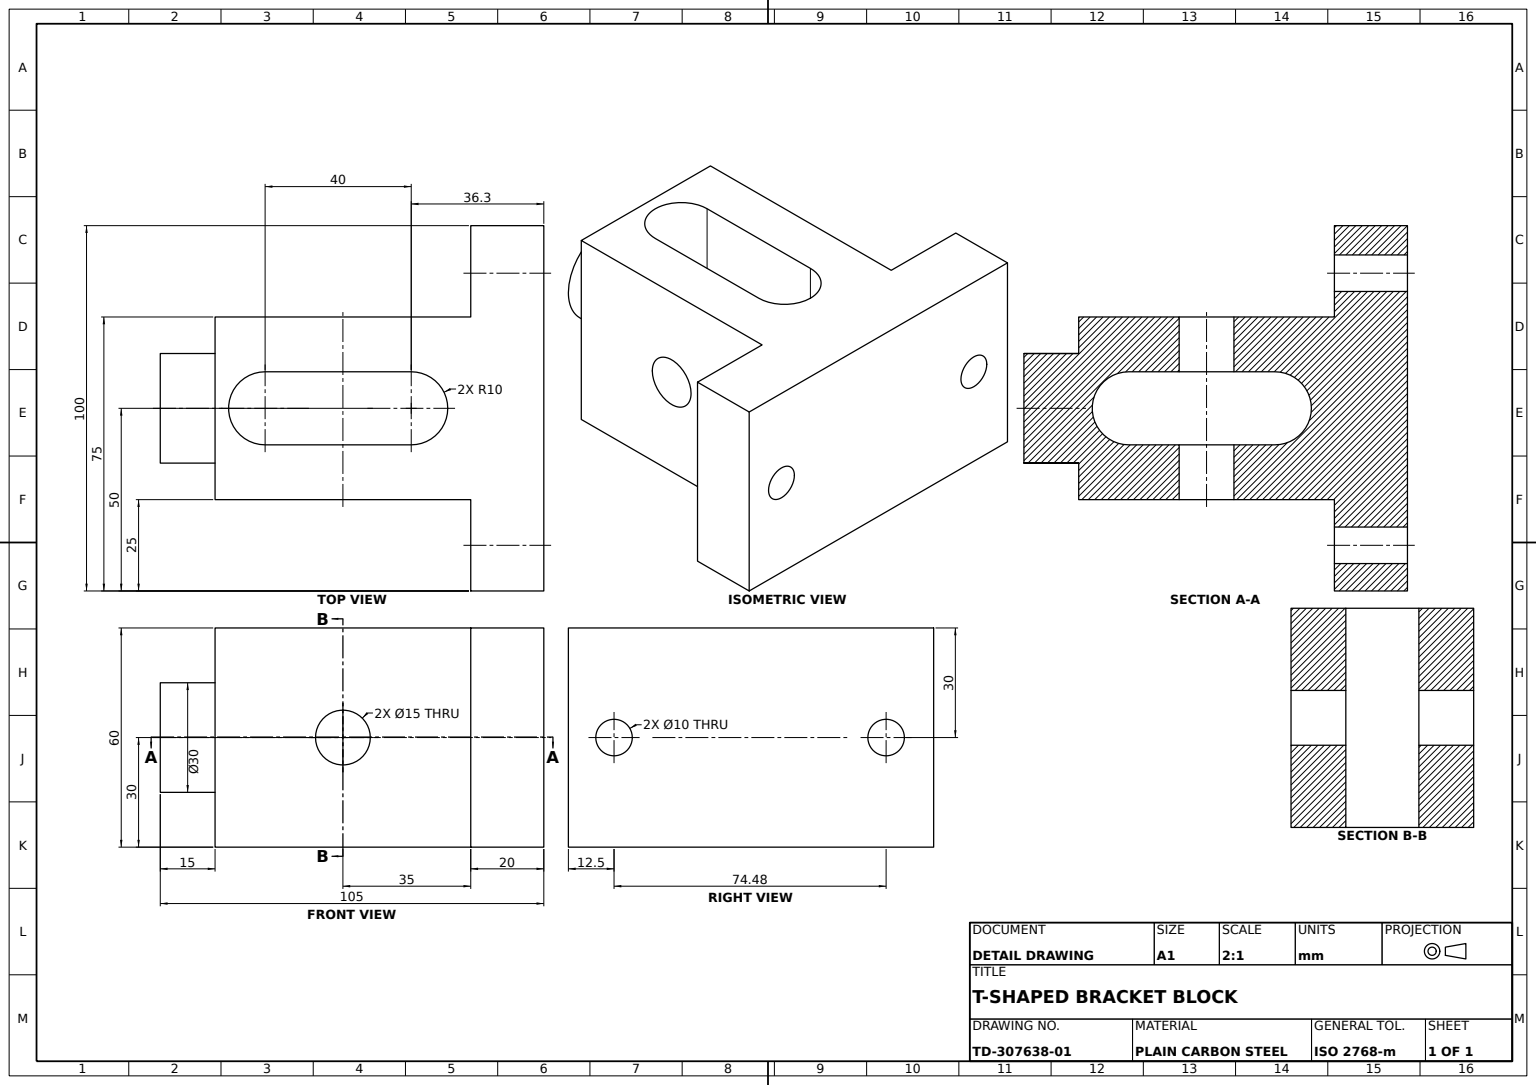
SolidWorks part; units mm, degrees
material "Plain Carbon Steel"
ref_plane "Front Plane" through (0, 0, 0) normal (0, 0, 1) x (1, 0, 0)
ref_plane "Top Plane" through (0, 0, 0) normal (0, 1, 0) x (1, 0, 0)
ref_plane "Right Plane" through (0, 0, 0) normal (1, 0, 0) x (0, 0, -1)
sketch "Base Plate Sketch" plane through (0, 0, 0) normal (0, 0, 1) x (1, 0, 0)
  line L0 (0, 0) -> (100, 0)
  line L1 (100, 0) -> (100, 60)
  line L2 (100, 60) -> (0, 60)
  line L3 (0, 60) -> (0, 0)
  dimension "D1" = 100
  dimension "D2" = 60
extrude "Base Plate" add sketch "Base Plate Sketch" along normal blind 20
sketch "Upright Block Sketch" plane through (0, 0, 0) normal (0, -1, 0) x (1, 0, 0)
  line L0 (50, 20) -> (25, 20)
  line L1 (100, 20) -> (100, 0) construction
  line L5 (0, 20) -> (100, 20) construction
  line L7 (25, 20) -> (25, 90)
  line L8 (25, 90) -> (75, 90)
  line L9 (75, 90) -> (75, 20)
  line L10 (75, 20) -> (50, 20)
  line L11 (0, 0) -> (100, 0) construction
  dimension "D1" = 25
  dimension "D2" = 90
extrude "Upright Block" add sketch "Upright Block Sketch" against normal blind 60
sketch "Top Slot Sketch" plane through (0, 0, 0) normal (0, -1, 0) x (1, 0, 0)
  line L0 (25, 90) -> (25, 20) construction
  line L1 (75, 20) -> (75, 90) construction
  line L2 (40, 76.2973) -> (40, 36.2973)
  line L4 (60, 36.2973) -> (60, 76.2973)
  arc A0 (60, 76.2973) -> (40, 76.2973) centre (50, 76.2973) ccw
  arc A1 (40, 36.2973) -> (60, 36.2973) centre (50, 36.2973) ccw
  dimension "D1" = 40
  dimension "D5" = 10
  dimension "D2" = 25
  dimension "D3" = 25
  dimension "D4" = 25
  dimension "D6" = 36.2973
extrude "Top Slot" cut sketch "Top Slot Sketch" against normal blind 60
sketch "Notch Sketch" plane through (0, 0, 20) normal (0, 0, 1) x (1, 0, 0)
  line L0 (75, 60) -> (75, 0) construction
  line L1 (100, 60) -> (75, 60) construction
  circle A0 centre (87.5, 30) radius 5
  circle A1 centre (13.0162, 30) radius 5
  dimension "D1" = 10
  dimension "D2" = 12.5
  dimension "D3" = 61.9838
  dimension "D4" = 30
extrude "Notch Cut" cut sketch "Notch Sketch" against normal blind 20
sketch "Cross Hole A Ø15 Sketch" plane through (75, 0, 0) normal (1, 0, 0) x (0, 0, -1)
  line L0 (-20, 0) -> (-90, 0) construction
  circle A0 centre (-55, 30) radius 7.5
  dimension "D1" = 15
  dimension "D2" = 15
  dimension "D3" = 35
  dimension "D4" = 30
extrude "Cross Hole A Ø15" cut sketch "Cross Hole A Ø15 Sketch" against normal blind 25
sketch "Cross Hole B Ø15 Sketch" plane through (25, 0, 0) normal (-1, 0, 0) x (0, 0, 1)
  line L0 (90, 0) -> (20, 0) construction
  circle A0 centre (55, 30) radius 7.5
  dimension "D1" = 15
  dimension "D2" = 15
  dimension "D3" = 35
  dimension "D4" = 30
extrude "Cross Hole B Ø15" cut sketch "Cross Hole B Ø15 Sketch" against normal blind 25
sketch "Pin Boss Ø30 Sketch" plane through (0, 0, 90) normal (0, 0, 1) x (1, 0, 0)
  line L0 (75, 60) -> (75, 0) construction
  line L1 (75, 0) -> (25, 0) construction
  circle A0 centre (50, 30) radius 15
  dimension "D1" = 30
  dimension "D2" = 30
  dimension "D3" = 25
  dimension "D4" = 30
extrude "Pin Boss Ø30" add sketch "Pin Boss Ø30 Sketch" along normal blind 15
